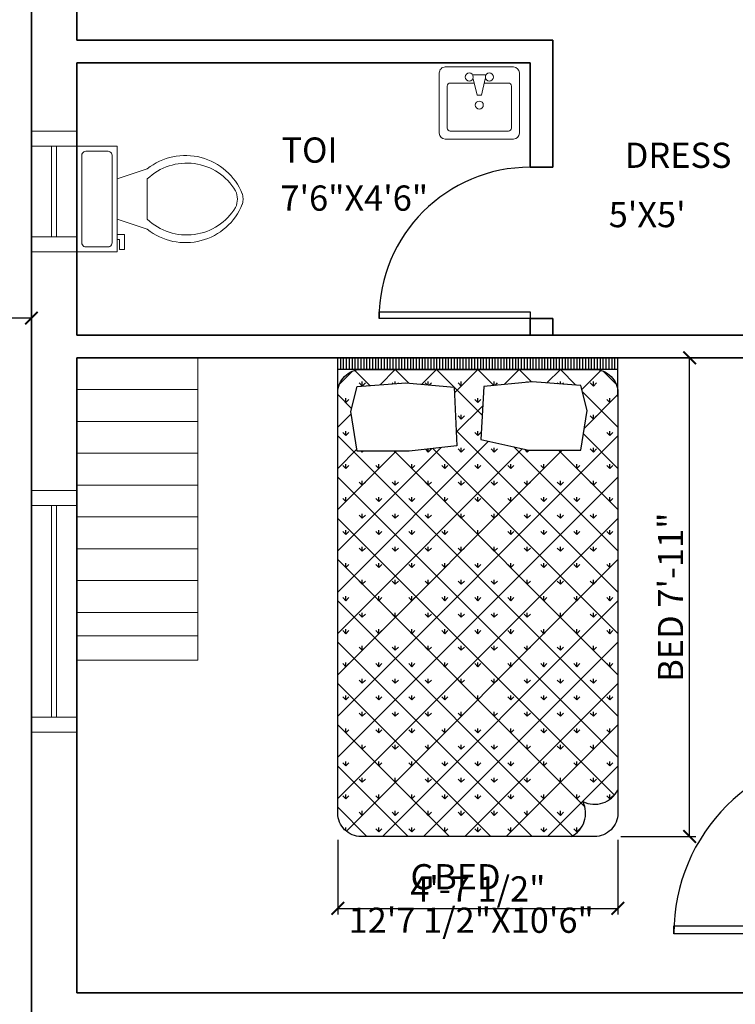
# Model space of a CAD drawing. Units: inches. Extents: x 3283068 to 3284536, y 3240756 to 3241803.
# Tile 5 of 19: x 3283337 to 3283479, y 3241305 to 3241501. Entities that reach past the tile are written whole.
import ezdxf

# ---------------------------------------------------------------- set-up
doc = ezdxf.new("R2010")
doc.units = ezdxf.units.IN
for name, color, linetype, lineweight in [('A-ANNO-DIMS', 2, 'Continuous', 18), ('A-AREA-IDEN', 7, 'Continuous', 18), ('A-FLOR-FIXT', 9, 'Continuous', 18), ('door', 140, 'Continuous', 25), ('furniture', 40, 'Continuous', 18), ('wall', 20, 'Continuous', 35), ('wardrobe', 180, 'Continuous', 18), ('window', 100, 'Continuous', 18)]:
    doc.layers.add(name, color=color, linetype=linetype, lineweight=lineweight)
doc.layers.add('NOI THAT', color=42, linetype='Continuous')
doc.styles.get("Standard").update_dxf_attribs({"font": 'arial.ttf'})
doc.dimstyles.new('ISO-25', dxfattribs={"dimtxt": 5, "dimasz": 2.5, "dimexe": 1.25, "dimexo": 0.625, "dimtad": 1, "dimlunit": 4, "dimtxsty": 'Standard', "dimblk": 'ARCHTICK', "dimcen": 2.5, "dimadec": 0, "dimazin": 0, "dimtfac": 1, "dimtmove": 0, "dimatfit": 3, "dimfxl": 1, "dimarcsym": 0})

# ---------------------------------------------------------------- blocks, each defined once
blk = doc.blocks.new('_ArchTick')
at = {"color": 0, "linetype": 'ByBlock', "const_width": 0.15}
blk.add_lwpolyline([(-0.5, -0.5), (0.5, 0.5)], dxfattribs=at)
blk = doc.blocks.new('*D1')
at = {"layer": 'A-ANNO-DIMS', "color": 0, "lineweight": -2, "transparency": 16777216}
for p, q in [((3283338.96, 3241639.1), (3283304.8, 3241639.1)), ((3283306.05, 3241198.1), (3283306.05, 3241639.1)), ((3283338.96, 3241198.1), (3283304.8, 3241198.1))]:
    blk.add_line(p, q, dxfattribs=at)
at = {"layer": 'Defpoints', "color": 0, "transparency": 16777216}
for p in [(3283306.05, 3241639.1), (3283339.59, 3241639.1), (3283339.59, 3241198.1)]:
    blk.add_point(p, dxfattribs=at)
at = {"layer": 'A-ANNO-DIMS', "color": 0, "lineweight": -2, "transparency": 16777216, "xscale": 2.5, "yscale": 2.5, "zscale": 2.5}
for p, rotation in [((3283306.05, 3241639.1), 90), ((3283306.05, 3241198.1), 270)]:
    blk.add_blockref('_ArchTick', p, dxfattribs=dict(at, rotation=rotation))
at = {"layer": 'A-ANNO-DIMS', "color": 0, "transparency": 16777216, "insert": (3283302.87, 3241418.6), "char_height": 5, "attachment_point": 5, "rotation": 90}
blk.add_mtext('36\'-9"', dxfattribs=at)
blk = doc.blocks.new('*U5')
for p, q in [((-40, 0), (-40, 6)), ((0, 0), (0, 6))]:
    blk.add_line(p, q)
blk.add_lwpolyline([(0, 0), (0, -40), (-1.75, -40), (-1.75, 0)], close=True)
blk.add_arc((0, 0), 40, 180, 270)
blk = doc.blocks.new('*X15')
at = {"color": 0}
for p, q in [((-424.3, 0), (-424.3, 0)), ((-424.3, 0), (-424.3, 0)), ((-141.4, 0), (-141.4, 0)), ((-282.8, 0), (-282.8, 0)), ((-282.8, 0), (-282.8, 0)), ((282.8, 0), (282.8, 0)), ((424.3, 0), (424.3, 0)), ((-495.1, -70.6), (-508.2, -57.5)), ((-495, -70.6), (-495, -52)), ((-494.9, -70.6), (-481.7, -57.5)), ((-363.4, -60.9), (-366.8, -57.5)), ((-353.6, -60.2), (-353.6, -52)), ((-342.2, -59.3), (-340.3, -57.5)), ((-217.5, -65.3), (-225.4, -57.5)), ((-212.1, -65.8), (-212.1, -52)), ((-207.7, -66.2), (-198.9, -57.5)), ((-70.7, -70.7), (-84, -57.5)), ((-70.7, -70.7), (-70.7, -52)), ((-70.7, -70.7), (-57.5, -57.5)), ((68.3, -68.3), (57.5, -57.5)), ((70.7, -68.1), (70.7, -52)), ((73.6, -67.8), (84, -57.5)), ((212.1, -55), (212.1, -52)), ((344.1, -61.2), (340.3, -57.5)), ((353.6, -61.9), (353.6, -52)), ((361.7, -62.5), (366.8, -57.5)), ((495, -70.7), (481.7, -57.5)), ((495, -70.7), (495, -52)), ((495, -70.7), (508.2, -57.5)), ((-565.7, -141.4), (-565.7, -122.7)), ((0, -141.4), (0, -122.7)), ((565.7, -141.4), (565.7, -122.7)), ((-565.7, -141.4), (-578.9, -128.2)), ((-565.7, -141.4), (-552.4, -128.2)), ((0, -141.4), (-13.3, -128.2)), ((0, -141.4), (13.3, -128.2)), ((565.7, -141.4), (552.4, -128.2)), ((565.7, -141.4), (578.9, -128.2)), ((-70.7, -212.1), (-84, -198.9)), ((-70.7, -212.1), (-70.7, -193.4)), ((-70.7, -212.1), (-57.5, -198.9)), ((495, -212.1), (481.7, -198.9)), ((495, -212.1), (495, -193.4)), ((495, -212.1), (508.2, -198.9)), ((-565.7, -282.8), (-578.9, -269.6)), ((-565.7, -282.8), (-565.7, -264.1)), ((-565.7, -282.8), (-552.4, -269.6)), ((0, -282.8), (-13.3, -269.6)), ((0, -282.8), (0, -264.1)), ((0, -282.8), (13.3, -269.6)), ((565.7, -282.8), (552.4, -269.6)), ((565.7, -282.8), (565.7, -264.1)), ((565.7, -282.8), (578.9, -269.6)), ((-70.7, -353.6), (-70.7, -334.8)), ((70.7, -353.6), (70.7, -334.8)), ((495, -353.6), (495, -334.8)), ((-495, -353.6), (-499, -349.5)), ((-495, -353.6), (-495, -349.5)), ((-495, -353.6), (-491, -349.5)), ((-353.6, -353.6), (-357.6, -349.5)), ((-353.6, -353.6), (-353.6, -349.5)), ((-353.6, -353.6), (-349.5, -349.5)), ((-212.1, -353.6), (-224, -341.7)), ((-212.1, -353.6), (-212.1, -340.3)), ((-212.1, -353.6), (-198.9, -340.3)), ((-70.7, -353.6), (-84, -340.3)), ((-70.7, -353.6), (-57.5, -340.3)), ((70.7, -353.6), (57.5, -340.3)), ((70.7, -353.6), (84, -340.3)), ((212.1, -353.6), (200.4, -341.8)), ((212.1, -353.6), (212.1, -344.4)), ((212.1, -353.6), (220, -345.7)), ((353.6, -353.6), (345.7, -345.7)), ((353.6, -353.6), (353.6, -345.7)), ((353.6, -353.6), (361.4, -345.7)), ((495, -353.6), (481.7, -340.3)), ((495, -353.6), (508.2, -340.3)), ((-565.7, -424.3), (-578.9, -411)), ((-565.7, -424.3), (-565.7, -405.5)), ((-565.7, -424.3), (-552.4, -411)), ((-424.3, -424.3), (-437.5, -411)), ((-424.3, -424.3), (-424.3, -405.5)), ((-424.3, -424.3), (-411, -411)), ((-282.8, -424.3), (-296.1, -411)), ((-282.8, -424.3), (-282.8, -405.5)), ((-282.8, -424.3), (-269.6, -411)), ((-141.4, -424.3), (-154.7, -411)), ((-141.4, -424.3), (-141.4, -405.5)), ((-141.4, -424.3), (-128.2, -411)), ((0, -424.3), (-13.3, -411)), ((0, -424.3), (0, -405.5)), ((0, -424.3), (13.3, -411)), ((141.4, -424.3), (128.2, -411)), ((141.4, -424.3), (141.4, -405.5)), ((141.4, -424.3), (154.7, -411)), ((282.8, -424.3), (269.6, -411)), ((282.8, -424.3), (282.8, -405.5)), ((282.8, -424.3), (296.1, -411)), ((424.3, -424.3), (411, -411)), ((424.3, -424.3), (424.3, -405.5)), ((424.3, -424.3), (437.5, -411)), ((565.7, -424.3), (552.4, -411)), ((565.7, -424.3), (565.7, -405.5)), ((565.7, -424.3), (578.9, -411)), ((-495, -495), (-508.2, -481.7)), ((-495, -495), (-495, -476.2)), ((-495, -495), (-481.7, -481.7)), ((-353.6, -495), (-366.8, -481.7)), ((-353.6, -495), (-353.6, -476.2)), ((-353.6, -495), (-340.3, -481.7)), ((-212.1, -495), (-225.4, -481.7)), ((-212.1, -495), (-212.1, -476.2)), ((-212.1, -495), (-198.9, -481.7)), ((-70.7, -495), (-84, -481.7)), ((-70.7, -495), (-70.7, -476.2)), ((-70.7, -495), (-57.5, -481.7)), ((70.7, -495), (57.5, -481.7)), ((70.7, -495), (70.7, -476.2)), ((70.7, -495), (84, -481.7)), ((212.1, -495), (198.9, -481.7)), ((212.1, -495), (212.1, -476.2)), ((212.1, -495), (225.4, -481.7)), ((353.6, -495), (340.3, -481.7)), ((353.6, -495), (353.6, -476.2)), ((353.6, -495), (366.8, -481.7)), ((495, -495), (481.7, -481.7)), ((495, -495), (495, -476.2)), ((495, -495), (508.2, -481.7)), ((-565.7, -565.7), (-565.7, -546.9)), ((-424.3, -565.7), (-424.3, -546.9)), ((-282.8, -565.7), (-282.8, -546.9)), ((-141.4, -565.7), (-141.4, -546.9)), ((0, -565.7), (0, -546.9)), ((141.4, -565.7), (141.4, -546.9)), ((282.8, -565.7), (282.8, -546.9)), ((424.3, -565.7), (424.3, -546.9)), ((565.7, -565.7), (565.7, -546.9)), ((-565.7, -565.7), (-578.9, -552.4)), ((-565.7, -565.7), (-552.4, -552.4)), ((-424.3, -565.7), (-437.5, -552.4)), ((-424.3, -565.7), (-411, -552.4)), ((-282.8, -565.7), (-296.1, -552.4)), ((-282.8, -565.7), (-269.6, -552.4)), ((-141.4, -565.7), (-154.7, -552.4)), ((-141.4, -565.7), (-128.2, -552.4)), ((0, -565.7), (-13.3, -552.4)), ((0, -565.7), (13.3, -552.4)), ((141.4, -565.7), (128.2, -552.4)), ((141.4, -565.7), (154.7, -552.4)), ((282.8, -565.7), (269.6, -552.4)), ((282.8, -565.7), (296.1, -552.4)), ((424.3, -565.7), (411, -552.4)), ((424.3, -565.7), (437.5, -552.4)), ((565.7, -565.7), (552.4, -552.4)), ((565.7, -565.7), (578.9, -552.4)), ((-495, -636.4), (-508.2, -623.1)), ((-495, -636.4), (-495, -617.6)), ((-495, -636.4), (-481.7, -623.1)), ((-353.6, -636.4), (-366.8, -623.1)), ((-353.6, -636.4), (-353.6, -617.6)), ((-353.6, -636.4), (-340.3, -623.1)), ((-212.1, -636.4), (-225.4, -623.1)), ((-212.1, -636.4), (-212.1, -617.6)), ((-212.1, -636.4), (-198.9, -623.1)), ((-70.7, -636.4), (-84, -623.1)), ((-70.7, -636.4), (-70.7, -617.6)), ((-70.7, -636.4), (-57.5, -623.1)), ((70.7, -636.4), (57.5, -623.1)), ((70.7, -636.4), (70.7, -617.6)), ((70.7, -636.4), (84, -623.1)), ((212.1, -636.4), (198.9, -623.1)), ((212.1, -636.4), (212.1, -617.6)), ((212.1, -636.4), (225.4, -623.1)), ((353.6, -636.4), (340.3, -623.1)), ((353.6, -636.4), (353.6, -617.6)), ((353.6, -636.4), (366.8, -623.1)), ((495, -636.4), (481.7, -623.1)), ((495, -636.4), (495, -617.6)), ((495, -636.4), (508.2, -623.1)), ((-565.7, -707.1), (-578.9, -693.8)), ((-565.7, -707.1), (-565.7, -688.4)), ((-565.7, -707.1), (-552.4, -693.8)), ((-424.3, -707.1), (-437.5, -693.8)), ((-424.3, -707.1), (-424.3, -688.4)), ((-424.3, -707.1), (-411, -693.8)), ((-282.8, -707.1), (-296.1, -693.8)), ((-282.8, -707.1), (-282.8, -688.4)), ((-282.8, -707.1), (-269.6, -693.8)), ((-141.4, -707.1), (-154.7, -693.8)), ((-141.4, -707.1), (-141.4, -688.4)), ((-141.4, -707.1), (-128.2, -693.8)), ((0, -707.1), (-13.3, -693.8)), ((0, -707.1), (0, -688.4)), ((0, -707.1), (13.3, -693.8)), ((141.4, -707.1), (128.2, -693.8)), ((141.4, -707.1), (141.4, -688.4)), ((141.4, -707.1), (154.7, -693.8)), ((282.8, -707.1), (269.6, -693.8)), ((282.8, -707.1), (282.8, -688.4)), ((282.8, -707.1), (296.1, -693.8)), ((424.3, -707.1), (411, -693.8)), ((424.3, -707.1), (424.3, -688.4)), ((424.3, -707.1), (437.5, -693.8)), ((565.7, -707.1), (552.4, -693.8)), ((565.7, -707.1), (565.7, -688.4)), ((565.7, -707.1), (578.9, -693.8)), ((-495, -777.8), (-508.2, -764.6)), ((-495, -777.8), (-495, -759.1)), ((-495, -777.8), (-481.7, -764.6)), ((-353.6, -777.8), (-366.8, -764.6)), ((-353.6, -777.8), (-353.6, -759.1)), ((-353.6, -777.8), (-340.3, -764.6)), ((-212.1, -777.8), (-225.4, -764.6)), ((-212.1, -777.8), (-212.1, -759.1)), ((-212.1, -777.8), (-198.9, -764.6)), ((-70.7, -777.8), (-84, -764.6)), ((-70.7, -777.8), (-70.7, -759.1)), ((-70.7, -777.8), (-57.5, -764.6)), ((70.7, -777.8), (57.5, -764.6)), ((70.7, -777.8), (70.7, -759.1)), ((70.7, -777.8), (84, -764.6)), ((212.1, -777.8), (198.9, -764.6)), ((212.1, -777.8), (212.1, -759.1)), ((212.1, -777.8), (225.4, -764.6)), ((353.6, -777.8), (340.3, -764.6)), ((353.6, -777.8), (353.6, -759.1)), ((353.6, -777.8), (366.8, -764.6)), ((495, -777.8), (481.7, -764.6)), ((495, -777.8), (495, -759.1)), ((495, -777.8), (508.2, -764.6)), ((-565.7, -848.5), (-578.9, -835.3)), ((-565.7, -848.5), (-565.7, -829.8)), ((-565.7, -848.5), (-552.4, -835.3)), ((-424.3, -848.5), (-437.5, -835.3)), ((-424.3, -848.5), (-424.3, -829.8)), ((-424.3, -848.5), (-411, -835.3)), ((-282.8, -848.5), (-296.1, -835.3)), ((-282.8, -848.5), (-282.8, -829.8)), ((-282.8, -848.5), (-269.6, -835.3)), ((-141.4, -848.5), (-154.7, -835.3)), ((-141.4, -848.5), (-141.4, -829.8)), ((-141.4, -848.5), (-128.2, -835.3)), ((0, -848.5), (-13.3, -835.3)), ((0, -848.5), (0, -829.8)), ((0, -848.5), (13.3, -835.3)), ((141.4, -848.5), (128.2, -835.3)), ((141.4, -848.5), (141.4, -829.8)), ((141.4, -848.5), (154.7, -835.3)), ((282.8, -848.5), (269.6, -835.3)), ((282.8, -848.5), (282.8, -829.8)), ((282.8, -848.5), (296.1, -835.3)), ((424.3, -848.5), (411, -835.3)), ((424.3, -848.5), (424.3, -829.8)), ((424.3, -848.5), (437.5, -835.3)), ((565.7, -848.5), (552.4, -835.3)), ((565.7, -848.5), (565.7, -829.8)), ((565.7, -848.5), (578.9, -835.3)), ((-495, -919.2), (-508.2, -906)), ((-495, -919.2), (-495, -900.5)), ((-495, -919.2), (-481.7, -906)), ((-353.6, -919.2), (-366.8, -906)), ((-353.6, -919.2), (-353.6, -900.5)), ((-353.6, -919.2), (-340.3, -906)), ((-212.1, -919.2), (-225.4, -906)), ((-212.1, -919.2), (-212.1, -900.5)), ((-212.1, -919.2), (-198.9, -906)), ((-70.7, -919.2), (-84, -906)), ((-70.7, -919.2), (-70.7, -900.5)), ((-70.7, -919.2), (-57.5, -906)), ((70.7, -919.2), (57.5, -906)), ((70.7, -919.2), (70.7, -900.5)), ((70.7, -919.2), (84, -906)), ((212.1, -919.2), (198.9, -906)), ((212.1, -919.2), (212.1, -900.5)), ((212.1, -919.2), (225.4, -906)), ((353.6, -919.2), (340.3, -906)), ((353.6, -919.2), (353.6, -900.5)), ((353.6, -919.2), (366.8, -906)), ((495, -919.2), (481.7, -906)), ((495, -919.2), (495, -900.5)), ((495, -919.2), (508.2, -906)), ((-565.7, -989.9), (-578.9, -976.7)), ((-565.7, -989.9), (-565.7, -971.2)), ((-565.7, -989.9), (-552.4, -976.7)), ((-424.3, -989.9), (-437.5, -976.7)), ((-424.3, -989.9), (-424.3, -971.2)), ((-424.3, -989.9), (-411, -976.7)), ((-282.8, -989.9), (-296.1, -976.7)), ((-282.8, -989.9), (-282.8, -971.2)), ((-282.8, -989.9), (-269.6, -976.7)), ((-141.4, -989.9), (-154.7, -976.7)), ((-141.4, -989.9), (-141.4, -971.2)), ((-141.4, -989.9), (-128.2, -976.7)), ((0, -989.9), (-13.3, -976.7)), ((0, -989.9), (0, -971.2)), ((0, -989.9), (13.3, -976.7)), ((141.4, -989.9), (128.2, -976.7)), ((141.4, -989.9), (141.4, -971.2)), ((141.4, -989.9), (154.7, -976.7)), ((282.8, -989.9), (269.6, -976.7)), ((282.8, -989.9), (282.8, -971.2)), ((282.8, -989.9), (296.1, -976.7)), ((424.3, -989.9), (411, -976.7)), ((424.3, -989.9), (424.3, -971.2)), ((424.3, -989.9), (437.5, -976.7)), ((565.7, -989.9), (552.4, -976.7)), ((565.7, -989.9), (565.7, -971.2)), ((565.7, -989.9), (578.9, -976.7)), ((-495, -1060.7), (-508.2, -1047.4)), ((-495, -1060.7), (-495, -1041.9)), ((-495, -1060.7), (-481.7, -1047.4)), ((-353.6, -1060.7), (-366.8, -1047.4)), ((-353.6, -1060.7), (-353.6, -1041.9)), ((-353.6, -1060.7), (-340.3, -1047.4)), ((-212.1, -1060.7), (-225.4, -1047.4)), ((-212.1, -1060.7), (-212.1, -1041.9)), ((-212.1, -1060.7), (-198.9, -1047.4)), ((-70.7, -1060.7), (-84, -1047.4)), ((-70.7, -1060.7), (-70.7, -1041.9)), ((-70.7, -1060.7), (-57.5, -1047.4)), ((70.7, -1060.7), (57.5, -1047.4)), ((70.7, -1060.7), (70.7, -1041.9)), ((70.7, -1060.7), (84, -1047.4)), ((212.1, -1060.7), (198.9, -1047.4)), ((212.1, -1060.7), (212.1, -1041.9)), ((212.1, -1060.7), (225.4, -1047.4)), ((353.6, -1060.7), (340.3, -1047.4)), ((353.6, -1060.7), (353.6, -1041.9)), ((353.6, -1060.7), (366.8, -1047.4)), ((495, -1060.7), (481.7, -1047.4)), ((495, -1060.7), (495, -1041.9)), ((495, -1060.7), (508.2, -1047.4)), ((-565.7, -1131.4), (-578.9, -1118.1)), ((-565.7, -1131.4), (-565.7, -1112.6)), ((-565.7, -1131.4), (-552.4, -1118.1)), ((-424.3, -1131.4), (-437.5, -1118.1)), ((-424.3, -1131.4), (-424.3, -1112.6)), ((-424.3, -1131.4), (-411, -1118.1)), ((-282.8, -1131.4), (-296.1, -1118.1)), ((-282.8, -1131.4), (-282.8, -1112.6)), ((-282.8, -1131.4), (-269.6, -1118.1)), ((-141.4, -1131.4), (-154.7, -1118.1)), ((-141.4, -1131.4), (-141.4, -1112.6)), ((-141.4, -1131.4), (-128.2, -1118.1)), ((0, -1131.4), (-13.3, -1118.1)), ((0, -1131.4), (0, -1112.6)), ((0, -1131.4), (13.3, -1118.1)), ((141.4, -1131.4), (128.2, -1118.1)), ((141.4, -1131.4), (141.4, -1112.6)), ((141.4, -1131.4), (154.7, -1118.1)), ((282.8, -1131.4), (269.6, -1118.1)), ((282.8, -1131.4), (282.8, -1112.6)), ((282.8, -1131.4), (296.1, -1118.1)), ((424.3, -1131.4), (411, -1118.1)), ((424.3, -1131.4), (424.3, -1112.6)), ((424.3, -1131.4), (437.5, -1118.1)), ((565.7, -1131.4), (552.4, -1118.1)), ((565.7, -1131.4), (565.7, -1112.6)), ((565.7, -1131.4), (578.9, -1118.1)), ((-495, -1202.1), (-508.2, -1188.8)), ((-495, -1202.1), (-495, -1183.3)), ((-495, -1202.1), (-481.7, -1188.8)), ((-353.6, -1202.1), (-366.8, -1188.8)), ((-353.6, -1202.1), (-353.6, -1183.3)), ((-353.6, -1202.1), (-340.3, -1188.8)), ((-212.1, -1202.1), (-225.4, -1188.8)), ((-212.1, -1202.1), (-212.1, -1183.3)), ((-212.1, -1202.1), (-198.9, -1188.8)), ((-70.7, -1202.1), (-84, -1188.8)), ((-70.7, -1202.1), (-70.7, -1183.3)), ((-70.7, -1202.1), (-57.5, -1188.8)), ((70.7, -1202.1), (57.5, -1188.8)), ((70.7, -1202.1), (70.7, -1183.3)), ((70.7, -1202.1), (84, -1188.8)), ((212.1, -1202.1), (198.9, -1188.8)), ((212.1, -1202.1), (212.1, -1183.3)), ((212.1, -1202.1), (225.4, -1188.8)), ((353.6, -1202.1), (340.3, -1188.8)), ((353.6, -1202.1), (353.6, -1183.3)), ((353.6, -1202.1), (366.8, -1188.8)), ((495, -1202.1), (481.7, -1188.8)), ((495, -1202.1), (495, -1183.3)), ((495, -1202.1), (508.2, -1188.8)), ((-565.7, -1272.8), (-578.9, -1259.5)), ((-565.7, -1272.8), (-565.7, -1254)), ((-565.7, -1272.8), (-552.4, -1259.5)), ((-424.3, -1272.8), (-437.5, -1259.5)), ((-424.3, -1272.8), (-424.3, -1254)), ((-424.3, -1272.8), (-411, -1259.5)), ((-282.8, -1272.8), (-296.1, -1259.5)), ((-282.8, -1272.8), (-282.8, -1254)), ((-282.8, -1272.8), (-269.6, -1259.5)), ((-141.4, -1272.8), (-154.7, -1259.5)), ((-141.4, -1272.8), (-141.4, -1254)), ((-141.4, -1272.8), (-128.2, -1259.5)), ((0, -1272.8), (-13.3, -1259.5)), ((0, -1272.8), (0, -1254)), ((0, -1272.8), (13.3, -1259.5)), ((141.4, -1272.8), (128.2, -1259.5)), ((141.4, -1272.8), (141.4, -1254)), ((141.4, -1272.8), (154.7, -1259.5)), ((282.8, -1272.8), (269.6, -1259.5)), ((282.8, -1272.8), (282.8, -1254)), ((282.8, -1272.8), (296.1, -1259.5)), ((424.3, -1272.8), (411, -1259.5)), ((424.3, -1272.8), (424.3, -1254)), ((424.3, -1272.8), (437.5, -1259.5)), ((565.7, -1272.8), (552.4, -1259.5)), ((565.7, -1272.8), (565.7, -1254)), ((565.7, -1272.8), (578.9, -1259.5)), ((-495, -1343.5), (-508.2, -1330.2)), ((-495, -1343.5), (-495, -1324.8)), ((-495, -1343.5), (-481.7, -1330.2)), ((-353.6, -1343.5), (-366.8, -1330.2)), ((-353.6, -1343.5), (-353.6, -1324.8)), ((-353.6, -1343.5), (-340.3, -1330.2)), ((-212.1, -1343.5), (-225.4, -1330.2)), ((-212.1, -1343.5), (-212.1, -1324.8)), ((-212.1, -1343.5), (-198.9, -1330.2)), ((-70.7, -1343.5), (-84, -1330.2)), ((-70.7, -1343.5), (-70.7, -1324.8)), ((-70.7, -1343.5), (-57.5, -1330.2)), ((70.7, -1343.5), (57.5, -1330.2)), ((70.7, -1343.5), (70.7, -1324.8)), ((70.7, -1343.5), (84, -1330.2)), ((212.1, -1343.5), (198.9, -1330.2)), ((212.1, -1343.5), (212.1, -1324.8)), ((212.1, -1343.5), (225.4, -1330.2)), ((353.6, -1343.5), (340.3, -1330.2)), ((353.6, -1343.5), (353.6, -1324.8)), ((353.6, -1343.5), (366.8, -1330.2)), ((495, -1343.5), (481.7, -1330.2)), ((495, -1343.5), (495, -1324.8)), ((495, -1343.5), (508.2, -1330.2)), ((-565.7, -1414.2), (-578.9, -1401)), ((-565.7, -1414.2), (-565.7, -1395.5)), ((-565.7, -1414.2), (-552.4, -1401)), ((-424.3, -1414.2), (-437.5, -1401)), ((-424.3, -1414.2), (-424.3, -1395.5)), ((-424.3, -1414.2), (-411, -1401)), ((-282.8, -1414.2), (-296.1, -1401)), ((-282.8, -1414.2), (-282.8, -1395.5)), ((-282.8, -1414.2), (-269.6, -1401)), ((-141.4, -1414.2), (-154.7, -1401)), ((-141.4, -1414.2), (-141.4, -1395.5)), ((-141.4, -1414.2), (-128.2, -1401)), ((0, -1414.2), (-13.3, -1401)), ((0, -1414.2), (0, -1395.5)), ((0, -1414.2), (13.3, -1401)), ((141.4, -1414.2), (128.2, -1401)), ((141.4, -1414.2), (141.4, -1395.5)), ((141.4, -1414.2), (154.7, -1401)), ((282.8, -1414.2), (269.6, -1401)), ((282.8, -1414.2), (282.8, -1395.5)), ((282.8, -1414.2), (296.1, -1401)), ((424.3, -1414.2), (411, -1401)), ((424.3, -1414.2), (424.3, -1395.5)), ((424.3, -1414.2), (437.5, -1401)), ((565.7, -1414.2), (552.4, -1401)), ((565.7, -1414.2), (565.7, -1395.5)), ((565.7, -1414.2), (578.9, -1401)), ((-495, -1484.9), (-508.2, -1471.7)), ((-495, -1484.9), (-495, -1466.2)), ((-495, -1484.9), (-481.7, -1471.7)), ((-353.6, -1484.9), (-366.8, -1471.7)), ((-353.6, -1484.9), (-353.6, -1466.2)), ((-353.6, -1484.9), (-340.3, -1471.7)), ((-212.1, -1484.9), (-225.4, -1471.7)), ((-212.1, -1484.9), (-212.1, -1466.2)), ((-212.1, -1484.9), (-198.9, -1471.7)), ((-70.7, -1484.9), (-84, -1471.7)), ((-70.7, -1484.9), (-70.7, -1466.2)), ((-70.7, -1484.9), (-57.5, -1471.7)), ((70.7, -1484.9), (57.5, -1471.7)), ((70.7, -1484.9), (70.7, -1466.2)), ((70.7, -1484.9), (84, -1471.7)), ((212.1, -1484.9), (198.9, -1471.7)), ((212.1, -1484.9), (212.1, -1466.2)), ((212.1, -1484.9), (225.4, -1471.7)), ((353.6, -1484.9), (340.3, -1471.7)), ((353.6, -1484.9), (353.6, -1466.2)), ((353.6, -1484.9), (366.8, -1471.7)), ((495, -1484.9), (481.7, -1471.7)), ((495, -1484.9), (495, -1466.2)), ((495, -1484.9), (508.2, -1471.7)), ((-565.7, -1555.6), (-578.9, -1542.4)), ((-565.7, -1555.6), (-565.7, -1536.9)), ((-565.7, -1555.6), (-552.4, -1542.4)), ((-424.3, -1555.6), (-437.5, -1542.4)), ((-424.3, -1555.6), (-424.3, -1536.9)), ((-424.3, -1555.6), (-411, -1542.4)), ((-282.8, -1555.6), (-296.1, -1542.4)), ((-282.8, -1555.6), (-282.8, -1536.9)), ((-282.8, -1555.6), (-269.6, -1542.4)), ((-141.4, -1555.6), (-154.7, -1542.4)), ((-141.4, -1555.6), (-141.4, -1536.9)), ((-141.4, -1555.6), (-128.2, -1542.4)), ((0, -1555.6), (-13.3, -1542.4)), ((0, -1555.6), (0, -1536.9)), ((0, -1555.6), (13.3, -1542.4)), ((141.4, -1555.6), (128.2, -1542.4)), ((141.4, -1555.6), (141.4, -1536.9)), ((141.4, -1555.6), (154.7, -1542.4)), ((282.8, -1555.6), (269.6, -1542.4)), ((282.8, -1555.6), (282.8, -1536.9)), ((282.8, -1555.6), (296.1, -1542.4)), ((424.3, -1555.6), (411, -1542.4)), ((424.3, -1555.6), (424.3, -1536.9)), ((424.3, -1555.6), (437.5, -1542.4)), ((565.7, -1555.6), (552.4, -1542.4)), ((565.7, -1555.6), (565.7, -1536.9)), ((565.7, -1555.6), (578.9, -1542.4)), ((-495, -1626.3), (-508.2, -1613.1)), ((-495, -1626.3), (-495, -1607.6)), ((-495, -1626.3), (-481.7, -1613.1)), ((-353.6, -1626.3), (-366.8, -1613.1)), ((-353.6, -1626.3), (-353.6, -1607.6)), ((-353.6, -1626.3), (-340.3, -1613.1)), ((-212.1, -1626.3), (-225.4, -1613.1)), ((-212.1, -1626.3), (-212.1, -1607.6)), ((-212.1, -1626.3), (-198.9, -1613.1)), ((-70.7, -1626.3), (-84, -1613.1)), ((-70.7, -1626.3), (-70.7, -1607.6)), ((-70.7, -1626.3), (-57.5, -1613.1)), ((70.7, -1626.3), (57.5, -1613.1)), ((70.7, -1626.3), (70.7, -1607.6)), ((70.7, -1626.3), (84, -1613.1)), ((212.1, -1626.3), (198.9, -1613.1)), ((212.1, -1626.3), (212.1, -1607.6)), ((212.1, -1626.3), (225.4, -1613.1)), ((353.6, -1626.3), (340.3, -1613.1)), ((353.6, -1626.3), (353.6, -1607.6)), ((353.6, -1626.3), (366.8, -1613.1)), ((495, -1626.3), (481.7, -1613.1)), ((495, -1626.3), (495, -1607.6)), ((495, -1626.3), (508.2, -1613.1)), ((-565.7, -1697.1), (-578.9, -1683.8)), ((-565.7, -1697.1), (-565.7, -1678.3)), ((-565.7, -1697.1), (-552.4, -1683.8)), ((-424.3, -1697.1), (-437.5, -1683.8)), ((-424.3, -1697.1), (-424.3, -1678.3)), ((-424.3, -1697.1), (-411, -1683.8)), ((-282.8, -1697.1), (-296.1, -1683.8)), ((-282.8, -1697.1), (-282.8, -1678.3)), ((-282.8, -1697.1), (-269.6, -1683.8)), ((-141.4, -1697.1), (-154.7, -1683.8)), ((-141.4, -1697.1), (-141.4, -1678.3)), ((-141.4, -1697.1), (-128.2, -1683.8)), ((0, -1697.1), (-13.3, -1683.8)), ((0, -1697.1), (0, -1678.3)), ((0, -1697.1), (13.3, -1683.8)), ((141.4, -1697.1), (128.2, -1683.8)), ((141.4, -1697.1), (141.4, -1678.3)), ((141.4, -1697.1), (154.7, -1683.8)), ((282.8, -1697.1), (269.6, -1683.8)), ((282.8, -1697.1), (282.8, -1678.3)), ((282.8, -1697.1), (296.1, -1683.8)), ((424.3, -1697.1), (411, -1683.8)), ((424.3, -1697.1), (424.3, -1678.3)), ((424.3, -1697.1), (437.5, -1683.8)), ((565.7, -1697.1), (552.4, -1683.8)), ((565.7, -1697.1), (565.7, -1678.3)), ((565.7, -1697.1), (578.9, -1683.8)), ((-495, -1767.8), (-508.2, -1754.5)), ((-495, -1767.8), (-495, -1749)), ((-495, -1767.8), (-481.7, -1754.5)), ((-353.6, -1767.8), (-366.8, -1754.5)), ((-353.6, -1767.8), (-353.6, -1749)), ((-353.6, -1767.8), (-340.3, -1754.5)), ((-212.1, -1767.8), (-225.4, -1754.5)), ((-212.1, -1767.8), (-212.1, -1749)), ((-212.1, -1767.8), (-198.9, -1754.5)), ((-70.7, -1767.8), (-84, -1754.5)), ((-70.7, -1767.8), (-70.7, -1749)), ((-70.7, -1767.8), (-57.5, -1754.5)), ((70.7, -1767.8), (57.5, -1754.5)), ((70.7, -1767.8), (70.7, -1749)), ((70.7, -1767.8), (84, -1754.5)), ((212.1, -1767.8), (198.9, -1754.5)), ((212.1, -1767.8), (212.1, -1749)), ((212.1, -1767.8), (225.4, -1754.5)), ((353.6, -1767.8), (340.3, -1754.5)), ((353.6, -1767.8), (353.6, -1749)), ((353.6, -1767.8), (366.8, -1754.5)), ((495, -1767.8), (481.7, -1754.5)), ((495, -1767.8), (495, -1749)), ((495, -1767.8), (508.2, -1754.5)), ((-565.7, -1838.5), (-578.9, -1825.2)), ((-565.7, -1838.5), (-565.7, -1819.7)), ((-565.7, -1838.5), (-552.4, -1825.2)), ((-424.3, -1838.5), (-437.5, -1825.2)), ((-424.3, -1838.5), (-424.3, -1819.7)), ((-424.3, -1838.5), (-411, -1825.2)), ((-282.8, -1838.5), (-296.1, -1825.2)), ((-282.8, -1838.5), (-282.8, -1819.7)), ((-282.8, -1838.5), (-269.6, -1825.2)), ((-141.4, -1838.5), (-154.7, -1825.2)), ((-141.4, -1838.5), (-141.4, -1819.7)), ((-141.4, -1838.5), (-128.2, -1825.2)), ((0, -1838.5), (-13.3, -1825.2)), ((0, -1838.5), (0, -1819.7)), ((0, -1838.5), (13.3, -1825.2)), ((141.4, -1838.5), (128.2, -1825.2)), ((141.4, -1838.5), (141.4, -1819.7)), ((141.4, -1838.5), (154.7, -1825.2)), ((282.8, -1838.5), (269.6, -1825.2)), ((282.8, -1838.5), (282.8, -1819.7)), ((282.8, -1838.5), (296.1, -1825.2)), ((424.3, -1838.5), (411, -1825.2)), ((424.3, -1838.5), (424.3, -1819.7)), ((424.3, -1838.5), (437.5, -1825.2)), ((565.7, -1838.5), (552.4, -1825.2)), ((565.7, -1838.5), (565.7, -1819.7)), ((565.7, -1838.5), (578.9, -1825.2)), ((-495, -1909.2), (-508.2, -1895.9)), ((-495, -1909.2), (-495, -1890.4)), ((-495, -1909.2), (-481.7, -1895.9)), ((-353.6, -1909.2), (-366.8, -1895.9)), ((-353.6, -1909.2), (-353.6, -1890.4)), ((-353.6, -1909.2), (-340.3, -1895.9)), ((-212.1, -1909.2), (-225.4, -1895.9)), ((-212.1, -1909.2), (-212.1, -1890.4)), ((-212.1, -1909.2), (-198.9, -1895.9)), ((-70.7, -1909.2), (-84, -1895.9)), ((-70.7, -1909.2), (-70.7, -1890.4)), ((-70.7, -1909.2), (-57.5, -1895.9)), ((70.7, -1909.2), (57.5, -1895.9)), ((70.7, -1909.2), (70.7, -1890.4)), ((70.7, -1909.2), (84, -1895.9)), ((212.1, -1909.2), (198.9, -1895.9)), ((212.1, -1909.2), (212.1, -1890.4)), ((212.1, -1909.2), (225.4, -1895.9)), ((353.6, -1909.2), (340.3, -1895.9)), ((353.6, -1909.2), (353.6, -1890.4)), ((353.6, -1909.2), (366.8, -1895.9)), ((-565.7, -1975.4), (-565.7, -1961.1)), ((-563.2, -1977.5), (-552.4, -1966.6)), ((-424.3, -1979.9), (-437.5, -1966.6)), ((-424.3, -1979.9), (-424.3, -1961.1)), ((-424.3, -1979.9), (-411, -1966.6)), ((-282.8, -1979.9), (-296.1, -1966.6)), ((-282.8, -1979.9), (-282.8, -1961.1)), ((-282.8, -1979.9), (-269.6, -1966.6)), ((-141.4, -1979.9), (-154.7, -1966.6)), ((-141.4, -1979.9), (-141.4, -1961.1)), ((-141.4, -1979.9), (-128.2, -1966.6)), ((0, -1979.9), (-13.3, -1966.6)), ((0, -1979.9), (0, -1961.1)), ((0, -1979.9), (13.3, -1966.6)), ((141.4, -1979.9), (128.2, -1966.6)), ((141.4, -1979.9), (141.4, -1961.1)), ((141.4, -1979.9), (154.7, -1966.6)), ((282.8, -1979.9), (269.6, -1966.6)), ((282.8, -1979.9), (282.8, -1961.1)), ((282.8, -1979.9), (296.1, -1966.6)), ((424.3, -1979.9), (411, -1966.6)), ((424.3, -1979.9), (424.3, -1961.1)), ((424.3, -1979.9), (437.5, -1966.6))]:
    blk.add_line(p, q, dxfattribs=at)
blk = doc.blocks.new('*X14')
at = {"color": 0}
for p, q in [((-592.6, -62.3), (-537.7, -7.4)), ((-462.1, -68.2), (-526.7, -3.6)), ((-418.5, -65), (-353.6, 0)), ((-295.4, -58.1), (-353.6, 0)), ((-240, -63.3), (-176.8, 0)), ((18.9, -195.7), (-176.8, 0)), ((-99.9, -99.9), (0, 0)), ((68.3, -68.3), (0, 0)), ((112.6, -64.2), (176.8, 0)), ((230.1, -53.3), (176.8, 0)), ((295.9, -57.6), (353.6, 0)), ((420.4, -66.9), (353.6, 0)), ((445.5, -84.9), (526.7, -3.6)), ((592.6, -62.3), (537.7, -7.4)), ((-540.7, -166.4), (-600, -107.1)), ((600, -246.4), (447.8, -94.3)), ((456.5, -250.6), (600, -107.1)), ((-92.1, -268.9), (21, -155.8)), ((-600, -246.4), (-542.7, -189.2)), ((-600, -1483.9), (600, -283.9)), ((600, -1483.9), (-600, -283.9)), ((600, -953.6), (-92.5, -261.1)), ((600, -423.2), (452.5, -275.7)), ((-600, -953.6), (46, -307.5)), ((-600, -776.8), (-157.3, -334.1)), ((600, -776.8), (154.9, -331.7)), ((-600, -1130.3), (190.7, -339.6)), ((-600, -423.2), (-518.4, -341.7)), ((-600, -1307.1), (361.4, -345.7)), ((-600, -600), (-349.5, -349.5)), ((600, -1307.1), (-357.6, -349.5)), ((600, -1130.3), (-192.3, -338.1)), ((600, -600), (345.7, -345.7)), ((-600, -1660.7), (600, -460.7)), ((600, -1660.7), (-600, -460.7)), ((-600, -1837.4), (600, -637.4)), ((585.1, -1822.5), (-600, -637.4)), ((458.4, -1872.6), (-600, -814.2)), ((-563.2, -1977.5), (600, -814.2)), ((405.9, -1996.8), (-600, -991)), ((-409, -2000), (600, -991)), ((232.2, -2000), (-600, -1167.8)), ((-232.2, -2000), (600, -1167.8)), ((55.5, -2000), (-600, -1344.5)), ((-55.5, -2000), (600, -1344.5)), ((-121.3, -2000), (-600, -1521.3)), ((121.3, -2000), (600, -1521.3)), ((-298.1, -2000), (-600, -1698.1)), ((298.1, -2000), (600, -1698.1)), ((-474.9, -2000), (-600, -1874.9))]:
    blk.add_line(p, q, dxfattribs=at)
blk = doc.blocks.new('*X16')
at = {"color": 0}
for p, q in [((-587.5, 0), (-587.5, 50)), ((-575, 0), (-575, 50)), ((-562.5, 0), (-562.5, 50)), ((-550, 0), (-550, 50)), ((-537.5, 0), (-537.5, 50)), ((-525, 0), (-525, 50)), ((-512.5, 0), (-512.5, 50)), ((-500, 0), (-500, 50)), ((-487.5, 0), (-487.5, 50)), ((-475, 0), (-475, 50)), ((-462.5, 0), (-462.5, 50)), ((-450, 0), (-450, 50)), ((-437.5, 0), (-437.5, 50)), ((-425, 0), (-425, 50)), ((-412.5, 0), (-412.5, 50)), ((-400, 0), (-400, 50)), ((-387.5, 0), (-387.5, 50)), ((-375, 0), (-375, 50)), ((-362.5, 0), (-362.5, 50)), ((-350, 0), (-350, 50)), ((-337.5, 0), (-337.5, 50)), ((-325, 0), (-325, 50)), ((-312.5, 0), (-312.5, 50)), ((-300, 0), (-300, 50)), ((-287.5, 0), (-287.5, 50)), ((-275, 0), (-275, 50)), ((-262.5, 0), (-262.5, 50)), ((-250, 0), (-250, 50)), ((-237.5, 0), (-237.5, 50)), ((-225, 0), (-225, 50)), ((-212.5, 0), (-212.5, 50)), ((-200, 0), (-200, 50)), ((-187.5, 0), (-187.5, 50)), ((-175, 0), (-175, 50)), ((-162.5, 0), (-162.5, 50)), ((-150, 0), (-150, 50)), ((-137.5, 0), (-137.5, 50)), ((-125, 0), (-125, 50)), ((-112.5, 0), (-112.5, 50)), ((-100, 0), (-100, 50)), ((-87.5, 0), (-87.5, 50)), ((-75, 0), (-75, 50)), ((-62.5, 0), (-62.5, 50)), ((-50, 0), (-50, 50)), ((-37.5, 0), (-37.5, 50)), ((-25, 0), (-25, 50)), ((-12.5, 0), (-12.5, 50)), ((0, 0), (0, 50)), ((12.5, 0), (12.5, 50)), ((25, 0), (25, 50)), ((37.5, 0), (37.5, 50)), ((50, 0), (50, 50)), ((62.5, 0), (62.5, 50)), ((75, 0), (75, 50)), ((87.5, 0), (87.5, 50)), ((100, 0), (100, 50)), ((112.5, 0), (112.5, 50)), ((125, 0), (125, 50)), ((137.5, 0), (137.5, 50)), ((150, 0), (150, 50)), ((162.5, 0), (162.5, 50)), ((175, 0), (175, 50)), ((187.5, 0), (187.5, 50)), ((200, 0), (200, 50)), ((212.5, 0), (212.5, 50)), ((225, 0), (225, 50)), ((237.5, 0), (237.5, 50)), ((250, 0), (250, 50)), ((262.5, 0), (262.5, 50)), ((275, 0), (275, 50)), ((287.5, 0), (287.5, 50)), ((300, 0), (300, 50)), ((312.5, 0), (312.5, 50)), ((325, 0), (325, 50)), ((337.5, 0), (337.5, 50)), ((350, 0), (350, 50)), ((362.5, 0), (362.5, 50)), ((375, 0), (375, 50)), ((387.5, 0), (387.5, 50)), ((400, 0), (400, 50)), ((412.5, 0), (412.5, 50)), ((425, 0), (425, 50)), ((437.5, 0), (437.5, 50)), ((450, 0), (450, 50)), ((462.5, 0), (462.5, 50)), ((475, 0), (475, 50)), ((487.5, 0), (487.5, 50)), ((500, 0), (500, 50)), ((512.5, 0), (512.5, 50)), ((525, 0), (525, 50)), ((537.5, 0), (537.5, 50)), ((550, 0), (550, 50)), ((562.5, 0), (562.5, 50)), ((575, 0), (575, 50)), ((587.5, 0), (587.5, 50))]:
    blk.add_line(p, q, dxfattribs=at)
blk = doc.blocks.new('A$C5BFD579E')
at = {"layer": 'NOI THAT'}
for p, q in [((0, 2050), (1200, 2050)), ((0, 1885.1), (0, 2050)), ((1200, 1885.1), (1200, 2050))]:
    blk.add_line(p, q, dxfattribs=at)
blk.add_lwpolyline([(100, 2000), (1100, 2000, -0.414214), (1200, 1900), (1200, 100, -0.414214), (1100, 0), (100, 0, -0.414214), (0, 100), (0, 1900, -0.414214)], format="xyb", close=True, dxfattribs=at)
blk.add_lwpolyline([(1200, 2000), (0, 2000)], dxfattribs=at)
for points in [[(290.9, 1943.1), (499, 1923.9), (510.6, 1673.6), (306.3, 1650.5), (82.8, 1650.5), (55.8, 1819.9), (82.8, 1927.7)], [(833.3, 1947), (625.2, 1927.7), (613.6, 1699.6), (817.9, 1654.3), (1041.4, 1654.3), (1068.3, 1823.8), (1041.4, 1931.6)]]:
    blk.add_lwpolyline(points, close=True, dxfattribs=at)
for centre, start, end in [((1100, 250), 243.4349, 333.4349), ((950, 100), 296.5651, 26.5651)]:
    blk.add_arc(centre, 111.8, start, end, dxfattribs=at)
for name in ['*X16', '*X14', '*X15']:
    blk.add_blockref(name, (600, 2000), dxfattribs=at)
blk = doc.blocks.new('*U22')
for p, q in [((241.3, -152.4), (241.3, -50.8)), ((-254, -215.9), (-203.2, -215.9)), ((-254, -241.3), (-254, -215.9)), ((-177.8, -241.3), (-254, -241.3)), ((-203.2, -215.9), (-203.2, -203.2)), ((-177.8, -203.2), (-177.8, -241.3)), ((-101.6, -203.2), (-152.4, -355.6)), ((101.6, -203.2), (152.4, -355.6)), ((101.6, -355.6), (-101.6, -355.6))]:
    blk.add_line(p, q)
blk.add_lwpolyline([(266.7, -203.2), (266.7, 0), (-266.7, 0), (-266.7, -203.2)], close=True)
for points in [[(215.9, -25.4), (-215.9, -25.4)], [(-241.3, -50.8), (-241.3, -152.4)], [(-215.9, -177.8), (215.9, -177.8)]]:
    blk.add_lwpolyline(points)
for centre, radius, start, end in [((-219.1, -47.6), 22.5, 81.8699, 188.1301), ((219.1, -47.6), 22.5, 351.8699, 98.1301), ((-219.1, -155.6), 22.5, 171.8699, 278.1301), ((219.1, -155.6), 22.5, 261.8699, 8.1301), ((89.4, -548.1), 309.1, 141.4691, 247.9714), ((106.7, -554.2), 287.8, 136.3677, 238.9468), ((-89.4, -548.1), 309.1, 292.0284, 38.5307), ((-106.7, -554.2), 287.8, 301.053, 43.6321), ((0, -708.1), 101.6, 245.7318, 294.2682), ((0, -736.6), 101.6, 254.8605, 285.1395)]:
    blk.add_arc(centre, radius, start, end)
blk = doc.blocks.new('*D26')
at = {"layer": 'A-ANNO-DIMS', "color": 0, "lineweight": -2, "transparency": 16777216}
for p, q in [((3283248.09, 3241434.23), (3283248.09, 3241442.74)), ((3283339.59, 3241441.49), (3283248.09, 3241441.49)), ((3283339.59, 3241434.23), (3283339.59, 3241442.74))]:
    blk.add_line(p, q, dxfattribs=at)
at = {"layer": 'Defpoints', "color": 0, "transparency": 16777216}
for p in [(3283248.09, 3241441.49), (3283248.09, 3241433.6), (3283339.59, 3241433.6)]:
    blk.add_point(p, dxfattribs=at)
at = {"layer": 'A-ANNO-DIMS', "color": 0, "lineweight": -2, "transparency": 16777216, "xscale": 2.5, "yscale": 2.5, "zscale": 2.5, "rotation": 180}
blk.add_blockref('_ArchTick', (3283248.09, 3241441.49), dxfattribs=at)
at = {"layer": 'A-ANNO-DIMS', "color": 0, "lineweight": -2, "transparency": 16777216, "xscale": 2.5, "yscale": 2.5, "zscale": 2.5}
blk.add_blockref('_ArchTick', (3283339.59, 3241441.49), dxfattribs=at)
at = {"layer": 'A-ANNO-DIMS', "color": 0, "transparency": 16777216, "insert": (3283293.84, 3241447.97), "char_height": 5, "attachment_point": 5}
blk.add_mtext('7\'-7{\\H1x;\\S1/2;}"', dxfattribs=at)
blk = doc.blocks.new('WIN-48IN-9IN-WALL')
for p, q in [((0, 9), (48, 9)), ((0, 0), (0, 9)), ((3, 0), (3, 9)), ((45, 9), (45, 0)), ((48, 9), (48, 0)), ((3, 5), (45, 5)), ((3, 4), (45, 4)), ((48, 0), (0, 0))]:
    blk.add_line(p, q)
blk = doc.blocks.new('LAVATORY-COMPACT')
for p, q in [((13.12, 15.9), (1.19, 15.9)), ((0, 14.71), (0, 1.19)), ((3.18, 8.94), (3.18, 13.71)), ((3.78, 14.31), (12.12, 14.31)), ((12.72, 13.71), (12.72, 2.19)), ((14.31, 1.19), (14.31, 14.71)), ((1.59, 6.76), (1.59, 9.14)), ((5.56, 8.35), (2.38, 9.14)), ((5.56, 7.55), (5.56, 8.35)), ((2.38, 6.76), (5.56, 7.55)), ((3.18, 2.19), (3.18, 6.96)), ((1.19, 0), (13.12, 0)), ((12.12, 1.59), (3.78, 1.59))]:
    blk.add_line(p, q)
for centre in [(1.99, 9.94), (7.55, 7.95), (1.99, 5.96)]:
    blk.add_circle(centre, 0.795)
for centre, radius, start, end in [((1.19, 14.71), 1.19, 90, 180), ((13.12, 14.71), 1.19, 0, 90), ((3.78, 13.71), 0.596, 90, 180), ((12.12, 13.71), 0.596, 0, 90), ((3.78, 2.19), 0.596, 180, 270), ((12.12, 2.19), 0.596, 270, 0), ((1.19, 1.19), 1.19, 180, 270), ((13.12, 1.19), 1.19, 270, 0)]:
    blk.add_arc(centre, radius, start, end)
blk = doc.blocks.new('WARDROBE-60X24IN')
for p, q in [((0, 53.69), (24, 53.69)), ((0, 47.37), (24, 47.37)), ((0, 41.06), (24, 41.06)), ((0, 34.75), (24, 34.75)), ((0, 28.44), (24, 28.44)), ((0, 22.12), (24, 22.12)), ((0, 15.81), (24, 15.81)), ((0, 9.5), (24, 9.5)), ((0, 4.82), (24, 4.82))]:
    blk.add_line(p, q)
blk.add_lwpolyline([(0, 60), (24, 60), (24, 0), (0, 0)], close=True)
blk = doc.blocks.new('*D47')
at = {"layer": 'A-ANNO-DIMS', "color": 0, "lineweight": -2, "transparency": 16777216}
for p, q in [((3283456.61, 3241433.6), (3283471.48, 3241433.6)), ((3283470.23, 3241338.63), (3283470.23, 3241433.6)), ((3283456.61, 3241338.63), (3283471.48, 3241338.63))]:
    blk.add_line(p, q, dxfattribs=at)
at = {"layer": 'Defpoints', "color": 0, "transparency": 16777216}
for p in [(3283455.99, 3241433.6), (3283470.23, 3241433.6), (3283455.99, 3241338.63)]:
    blk.add_point(p, dxfattribs=at)
at = {"layer": 'A-ANNO-DIMS', "color": 0, "lineweight": -2, "transparency": 16777216, "xscale": 2.5, "yscale": 2.5, "zscale": 2.5}
for p, rotation in [((3283470.23, 3241433.6), 90), ((3283470.23, 3241338.63), 270)]:
    blk.add_blockref('_ArchTick', p, dxfattribs=dict(at, rotation=rotation))
at = {"layer": 'A-ANNO-DIMS', "color": 0, "transparency": 16777216, "insert": (3283467.1, 3241386.12), "char_height": 5, "attachment_point": 5, "rotation": 90}
blk.add_mtext('BED 7\'-11"', dxfattribs=at)
blk = doc.blocks.new('*D48')
at = {"layer": 'A-ANNO-DIMS', "color": 0, "lineweight": -2, "transparency": 16777216}
for p, q in [((3283400.4, 3241338.01), (3283400.4, 3241323.14)), ((3283455.99, 3241338.01), (3283455.99, 3241323.14)), ((3283400.4, 3241324.39), (3283455.99, 3241324.39))]:
    blk.add_line(p, q, dxfattribs=at)
at = {"layer": 'Defpoints', "color": 0, "transparency": 16777216}
for p in [(3283400.4, 3241338.63), (3283455.99, 3241338.63), (3283455.99, 3241324.39)]:
    blk.add_point(p, dxfattribs=at)
at = {"layer": 'A-ANNO-DIMS', "color": 0, "lineweight": -2, "transparency": 16777216, "xscale": 2.5, "yscale": 2.5, "zscale": 2.5, "rotation": 180}
blk.add_blockref('_ArchTick', (3283400.4, 3241324.39), dxfattribs=at)
at = {"layer": 'A-ANNO-DIMS', "color": 0, "lineweight": -2, "transparency": 16777216, "xscale": 2.5, "yscale": 2.5, "zscale": 2.5}
blk.add_blockref('_ArchTick', (3283455.99, 3241324.39), dxfattribs=at)
at = {"layer": 'A-ANNO-DIMS', "color": 0, "transparency": 16777216, "insert": (3283428.19, 3241327.6), "char_height": 5, "attachment_point": 5}
blk.add_mtext('4\'-7 1/2"', dxfattribs=at)
blk = doc.blocks.new('*D63')
at = {"layer": 'A-ANNO-DIMS', "color": 0, "lineweight": -2, "transparency": 16777216}
for p, q in [((3283248.09, 3241083.23), (3283248.09, 3241798.08)), ((3283248.09, 3241796.83), (3284328.09, 3241796.83)), ((3284328.09, 3241083.23), (3284328.09, 3241798.08))]:
    blk.add_line(p, q, dxfattribs=at)
at = {"layer": 'Defpoints', "color": 0, "transparency": 16777216}
for p in [(3284328.09, 3241796.83), (3283248.09, 3241082.6), (3284328.09, 3241082.6)]:
    blk.add_point(p, dxfattribs=at)
at = {"layer": 'A-ANNO-DIMS', "color": 0, "lineweight": -2, "transparency": 16777216, "xscale": 2.5, "yscale": 2.5, "zscale": 2.5, "rotation": 180}
blk.add_blockref('_ArchTick', (3283248.09, 3241796.83), dxfattribs=at)
at = {"layer": 'A-ANNO-DIMS', "color": 0, "lineweight": -2, "transparency": 16777216, "xscale": 2.5, "yscale": 2.5, "zscale": 2.5}
blk.add_blockref('_ArchTick', (3284328.09, 3241796.83), dxfattribs=at)
at = {"layer": 'A-ANNO-DIMS', "color": 0, "transparency": 16777216, "insert": (3283788.09, 3241800.01), "char_height": 5, "attachment_point": 5}
blk.add_mtext('90\'-0"', dxfattribs=at)

msp = doc.modelspace()

# ---------------------------------------------------------------- linework, layer by layer
at = {"layer": 'door'}
for p, q in [((3283443.089, 3241471.417), (3283438.589, 3241471.417)), ((3283443.089, 3241441.417), (3283438.589, 3241441.417))]:
    msp.add_line(p, q, dxfattribs=at)
at = {"layer": 'wall'}
for p, q in [((3283339.589, 3241639.102), (3283339.589, 3241198.102)), ((3283348.589, 3241630.102), (3283348.589, 3241496.602)), ((3283443.089, 3241496.602), (3283348.589, 3241496.602)), ((3283443.089, 3241496.602), (3283443.089, 3241471.417)), ((3283348.589, 3241492.102), (3283438.589, 3241492.102)), ((3283348.589, 3241492.102), (3283438.589, 3241492.102)), ((3283348.589, 3241492.102), (3283348.589, 3241438.102)), ((3283348.589, 3241492.102), (3283348.589, 3241438.102)), ((3283438.589, 3241492.102), (3283438.589, 3241471.417)), ((3283438.589, 3241441.417), (3283438.589, 3241438.102)), ((3283443.089, 3241441.417), (3283443.089, 3241438.102)), ((3283348.589, 3241438.102), (3283503.089, 3241438.102)), ((3283348.589, 3241433.602), (3283503.089, 3241433.602)), ((3283348.589, 3241433.602), (3283348.589, 3241307.602)), ((3283348.589, 3241307.602), (3283503.089, 3241307.602))]:
    msp.add_line(p, q, dxfattribs=at)
at = {"layer": 'window'}
for p, q in [((3283339.589, 3241454.602), (3283339.589, 3241478.602)), ((3283339.589, 3241478.602), (3283348.589, 3241478.602)), ((3283348.589, 3241478.602), (3283348.589, 3241454.602)), ((3283339.589, 3241475.602), (3283348.589, 3241475.602)), ((3283343.589, 3241457.602), (3283343.589, 3241475.602)), ((3283344.589, 3241457.602), (3283344.589, 3241475.602)), ((3283348.589, 3241457.602), (3283339.589, 3241457.602)), ((3283348.589, 3241454.602), (3283339.589, 3241454.602))]:
    msp.add_line(p, q, dxfattribs=at)

# ---------------------------------------------------------------- block references
at = {"layer": 'A-FLOR-FIXT', "rotation": 269.9999999907282}
msp.add_blockref('LAVATORY-COMPACT', (3283420.54, 3241491.307), dxfattribs=at)
at = {"layer": 'A-FLOR-FIXT', "xscale": 0.0393700787401575, "yscale": 0.0393700787401575, "zscale": 0.0393700787401575, "rotation": 90}
msp.add_blockref('*U22', (3283348.589, 3241465.102), dxfattribs=at)
at = {"layer": 'door', "rotation": 270}
for p, xscale, yscale, zscale in [((3283438.589, 3241441.417), 0.75, 0.75, 0.75), ((3283503.089, 3241319.345), 0.9, 0.9, 0.9)]:
    msp.add_blockref('*U5', p, dxfattribs=dict(at, xscale=xscale, yscale=yscale, zscale=zscale))
at = {"layer": 'furniture', "xscale": 0.0463256999180216, "yscale": 0.0463256999180216, "zscale": 0.0463256999180216}
msp.add_blockref('A$C5BFD579E', (3283400.398, 3241338.635), dxfattribs=at)
at = {"layer": 'wardrobe'}
msp.add_blockref('WARDROBE-60X24IN', (3283348.589, 3241373.602), dxfattribs=at)
at = {"layer": 'window', "rotation": 270.0000000015438}
msp.add_blockref('WIN-48IN-9IN-WALL', (3283339.589, 3241407.309), dxfattribs=at)

# ---------------------------------------------------------------- texts
at = {"layer": 'A-AREA-IDEN'}
for s, p in [('TOI', (3283389.212, 3241472.321)), ('DRESS', (3283457.359, 3241471.29)), ('7\'6"X4\'6"', (3283389.014, 3241462.796)), ("5'X5'", (3283454.174, 3241459.522)), ('        GBED', (3283402.604, 3241328.159)), ('12\'7 1/2"X10\'6"', (3283402.553, 3241319.533))]:
    msp.add_text(s, height=5, dxfattribs=at).set_placement(p)

# ---------------------------------------------------------------- dimensions: what is measured, and where the dimension line sits
at = {"layer": 'A-ANNO-DIMS'}
for base, p1, p2, override, picture, middle in [((3284328.089, 3241796.827), (3283248.089, 3241082.602), (3284328.089, 3241082.602), {"dimdec": 1, "dimlfac": 1, "dimrnd": 0, "dimzin": 1, "dimdsep": 46, "dimlunit": 4, "dimfrac": 2}, '*D63', (3283788.089, 3241800.005)), ((3283248.089, 3241441.495), (3283339.589, 3241433.602), (3283248.089, 3241433.602), {"dimclrd": 0, "dimclre": 0, "dimclrt": 0}, '*D26', (3283293.839, 3241447.974)), ((3283455.989, 3241324.39), (3283400.398, 3241338.635), (3283455.989, 3241338.635), {"dimdec": 1, "dimlfac": 1, "dimrnd": 0, "dimzin": 1, "dimdsep": 46, "dimlunit": 4, "dimfrac": 2}, '*D48', (3283428.194, 3241327.6))]:
    dim = msp.add_linear_dim(base=base, p1=p1, p2=p2, dimstyle='ISO-25', override=override, dxfattribs=at)
    dim.commit()
    dim.dimension.update_dxf_attribs({"geometry": picture, "text_midpoint": middle})
dim = msp.add_linear_dim(base=(3283306.051, 3241639.102), p1=(3283339.589, 3241198.102), p2=(3283339.589, 3241639.102), angle=90, dimstyle='ISO-25', override={"dimclrd": 0, "dimclre": 0, "dimclrt": 0}, dxfattribs=at)
dim.commit()
dim.dimension.update_dxf_attribs({"geometry": '*D1', "text_midpoint": (3283302.872, 3241418.602)})
dim = msp.add_linear_dim(base=(3283470.234, 3241433.602), p1=(3283455.989, 3241338.635), p2=(3283455.989, 3241433.602), angle=90, text='BED <>', dimstyle='ISO-25', override={"dimdec": 1, "dimlfac": 1, "dimrnd": 0, "dimzin": 1, "dimdsep": 46, "dimlunit": 4, "dimfrac": 2}, dxfattribs=at)
dim.commit()
dim.dimension.update_dxf_attribs({"geometry": '*D47', "text_midpoint": (3283467.097, 3241386.119)})

doc.saveas('drawing.dxf')
